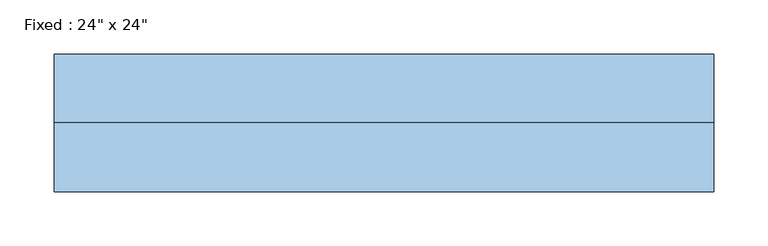
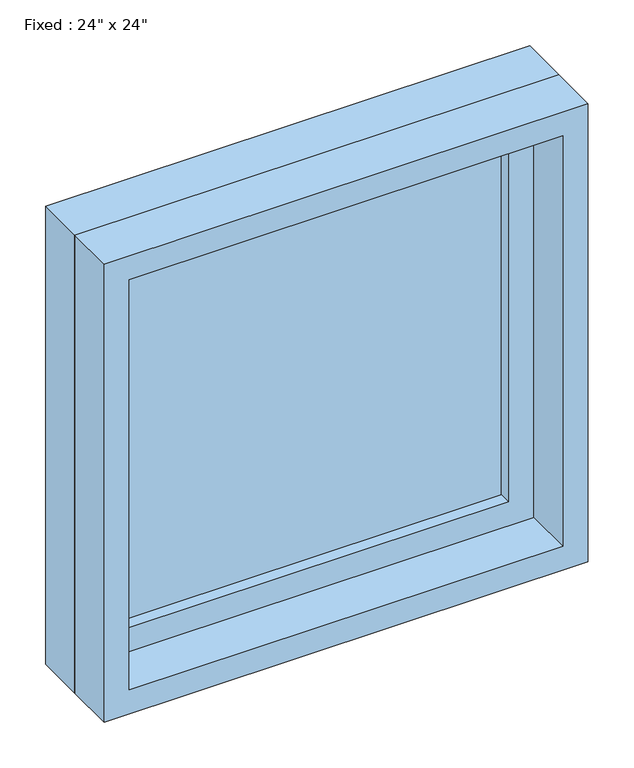
"""IFC4 building model written with IfcOpenShell, lengths in millimetres: window geometry."""

from ifc_helpers import new_model, si_unit, frame, origin, place, context, project, spatial, polyline, outline, extrude, source, transform, mapped, element, save


def window_d757e824(model_context):
    return source(origin(), model_context, "Body", "SweptSolid", [
        extrude(outline(polyline([(203.2, 15.875), (-279.4, 15.875), (-279.4, 28.575), (203.2, 28.575), (203.2, 15.875)])), frame((0.0, 0.0, 977.9), z_axis=(0.0, 0.0, 1.0), x_axis=(1.0, 0.0, 0.0)), (0.0, 0.0, 1.0), 482.6),
        extrude(outline(polyline([(1504.95, -323.85), (933.45, -323.85), (933.45, 247.65), (1504.95, 247.65), (1504.95, -323.85)]), holes=[polyline([(1460.5, -279.4), (1460.5, 203.2), (977.9, 203.2), (977.9, -279.4), (1460.5, -279.4)])]), frame((0.0, 0.0, 0.0), z_axis=(0.0, 1.0, 0.0), x_axis=(0.0, 0.0, 1.0)), (0.0, 0.0, 1.0), 44.45),
        extrude(outline(polyline([(1524.0, -342.9), (914.4, -342.9), (914.4, 266.7), (1524.0, 266.7), (1524.0, -342.9)]), holes=[polyline([(1492.25, -311.15), (1492.25, 234.95), (946.15, 234.95), (946.15, -311.15), (1492.25, -311.15)])]), frame((0.0, -63.5, 0.0), z_axis=(0.0, 1.0, 0.0), x_axis=(0.0, 0.0, 1.0)), (0.0, 0.0, 1.0), 63.5),
        extrude(outline(polyline([(1524.0, 266.7), (1524.0, -342.9), (914.4, -342.9), (914.4, 266.7), (1524.0, 266.7)]), holes=[polyline([(1504.95, 247.65), (933.45, 247.65), (933.45, -323.85), (1504.95, -323.85), (1504.95, 247.65)])]), frame((0.0, 0.0, 0.0), z_axis=(0.0, 1.0, 0.0), x_axis=(0.0, 0.0, 1.0)), (0.0, 0.0, 1.0), 63.5),
    ])


if __name__ == "__main__":
    model = new_model("IFC4")
    model_context = context("Model", 3, world=origin())
    ifc_project = project(units=[si_unit("LENGTHUNIT", "METRE", prefix="MILLI")], contexts=[model_context])
    site = spatial("IfcSite", under=ifc_project)
    building = spatial("IfcBuilding", under=site)
    placement = place(None, origin())
    window_shape = window_d757e824(model_context)
    element("IfcWindow", 1, ObjectType="Fixed : 24\" x 24\"", at=placement, inside=building, context=model_context, shape_type="MappedRepresentation", body=[
        mapped(window_shape, transform((0.0, 0.0, 0.0), x_axis=(1.0, 0.0, 0.0), y_axis=(0.0, 1.0, 0.0), z_axis=(0.0, 0.0, 1.0))),
    ])
    save(model, "model.ifc")

# Revit data of these elements
# Type "Fixed : 24\" x 24\""
#   Type Mark = "3"
#   Construction Type Id = "GSP4R"
#   Assembly Code = "B2020100"
#   Analytic Construction = "1/8 in Pilkington single glazing"
#   Visual Light Transmittance = 0.9
#   Solar Heat Gain Coefficient = 0.78
#   Heat Transfer Coefficient (U) = 0.6496 BTU/(h·ft²·°F)
#   Height = 2' - 0"
#   Default Sill Height = 3' - 0"
#   Width = 2' - 0"
#   Window Inset = 0' - 0 3/4"
#   Define Thermal Properties by = 1
#   Glass Pane Material = Glass
#   Sash Material = Sash
#   Wall Closure = (empty or 0)
# Element 1 (IfcWindow, "Fixed : 24\" x 24\"")
#   Materials on its faces: "Sash", "Glass"
# Materials
#   "Glass": class "Glass", colour RGB 0 128 192, transparency 0.75, Description = "Soda Lime Glass", Cost = 0
#   "Sash": class "Wood", colour RGB 224 178 126, transparency 0
